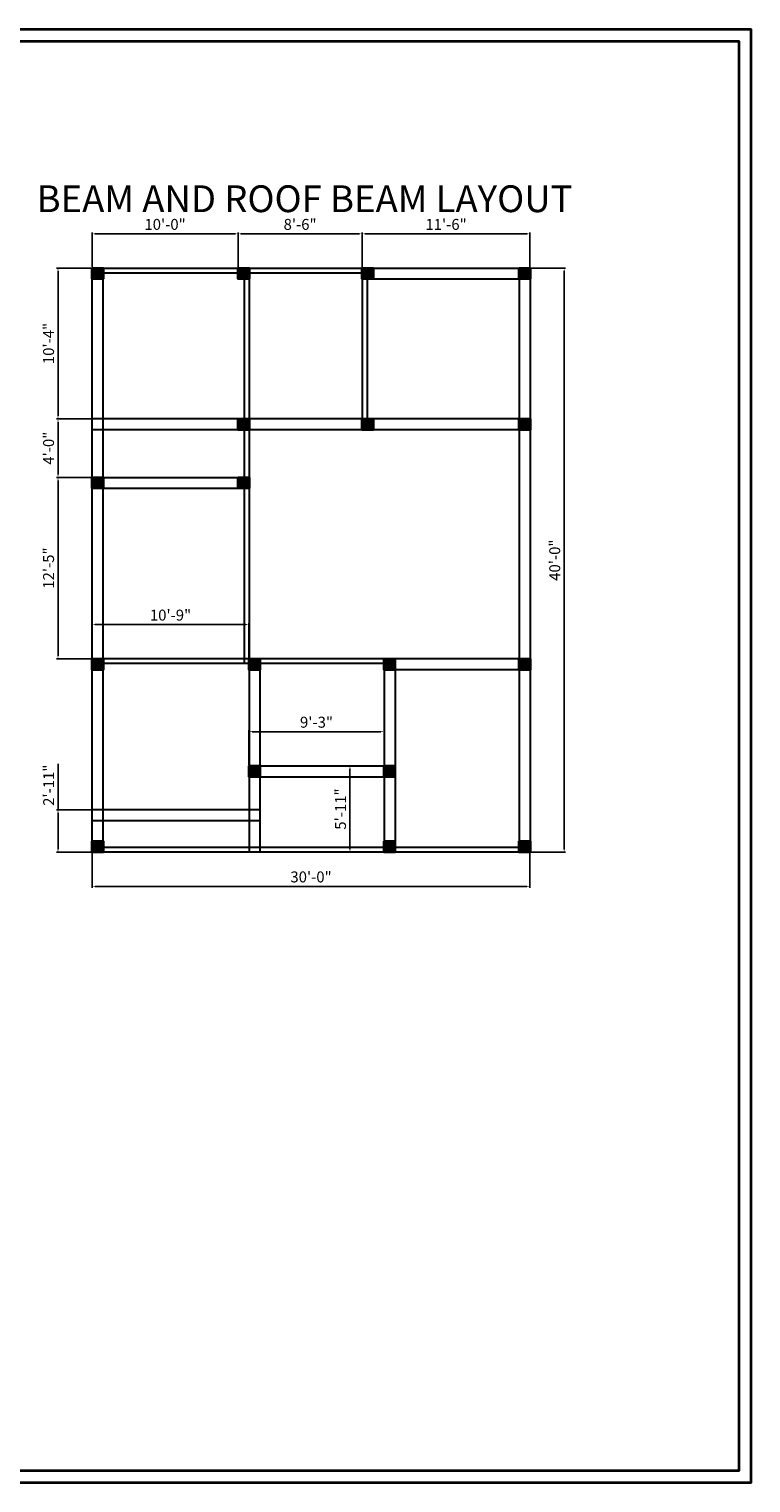
# Model space of a CAD drawing. Units: inches. Extents: x 2413 to 4117, y 1127 to 2321.
# Tile 5 of 5: x 3524 to 4117, y 1127 to 2321. Entities that reach past the tile are written whole.
import ezdxf

# ---------------------------------------------------------------- set-up
doc = ezdxf.new("R2010")
doc.units = ezdxf.units.IN
doc.linetypes.add('ACAD_ISO03W100', pattern=[30, 12, -18])
doc.layers.get('Defpoints').update_dxf_attribs({"linetype": 'ACAD_ISO03W100'})
for name, color, linetype, lineweight in [('A-ANNO-DIMS', 2, 'Continuous', 18), ('A-ANNO-TITL', 7, 'Continuous', 30), ('A-ANNO-TTLB', 7, 'Continuous', 35), ('S-BEAM', 3, 'Continuous', 30), ('S-COLS', 1, 'Continuous', 35)]:
    doc.layers.add(name, color=color, linetype=linetype, lineweight=lineweight)
doc.styles.get("Standard").update_dxf_attribs({"font": 'arial.ttf'})
doc.dimstyles.new('ISO-25', dxfattribs={"dimtxt": 9, "dimasz": 2.5, "dimexe": 1.25, "dimexo": 0.625, "dimgap": 2, "dimtad": 1, "dimdec": 1, "dimlunit": 4, "dimtxsty": 'Standard', "dimcen": 2.5, "dimazin": 0, "dimtfac": 1, "dimtdec": 1, "dimtmove": 0, "dimatfit": 3, "dimfxl": 1, "dimarcsym": 0})

# ---------------------------------------------------------------- blocks, each defined once
blk = doc.blocks.new('COLUMN')
h = blk.add_hatch(color=256)
h.dxf.hatch_style = 1
h.paths.add_polyline_path([(3657, 1935.4), (3666, 1935.4), (3666, 1944.4), (3657, 1944.4)])
blk.add_lwpolyline([(3657, 1944.4), (3666, 1944.4), (3666, 1935.4), (3657, 1935.4)], close=True)
blk = doc.blocks.new('*D54')
at = {"layer": 'A-ANNO-DIMS', "color": 0, "lineweight": -2, "transparency": 16777216}
for p, q in [((3575.4, 2125.7), (3575.4, 2154.3)), ((3577.9, 2153.1), (3692.9, 2153.1)), ((3695.4, 2125.7), (3695.4, 2154.3))]:
    blk.add_line(p, q, dxfattribs=at)
at = {"layer": 'A-ANNO-DIMS', "color": 0, "transparency": 16777216}
for points in [[(3577.9, 2153.5), (3577.9, 2152.7), (3575.4, 2153.1)], [(3692.9, 2153.5), (3692.9, 2152.7), (3695.4, 2153.1)]]:
    blk.add_solid(points, dxfattribs=at)
at = {"layer": 'Defpoints', "color": 0, "transparency": 16777216}
for p in [(3695.4, 2153.1), (3575.4, 2125), (3695.4, 2125)]:
    blk.add_point(p, dxfattribs=at)
at = {"layer": 'A-ANNO-DIMS', "color": 0, "transparency": 16777216, "insert": (3635.4, 2159.7), "char_height": 9, "attachment_point": 5}
blk.add_mtext('10\'-0"', dxfattribs=at)
blk = doc.blocks.new('*D55')
at = {"layer": 'A-ANNO-DIMS', "color": 0, "lineweight": -2, "transparency": 16777216}
for p, q in [((3695.4, 2125.7), (3695.4, 2154.3)), ((3697.9, 2153.1), (3794.9, 2153.1)), ((3797.4, 2125.7), (3797.4, 2154.3))]:
    blk.add_line(p, q, dxfattribs=at)
at = {"layer": 'A-ANNO-DIMS', "color": 0, "transparency": 16777216}
for points in [[(3697.9, 2153.5), (3697.9, 2152.7), (3695.4, 2153.1)], [(3794.9, 2153.5), (3794.9, 2152.7), (3797.4, 2153.1)]]:
    blk.add_solid(points, dxfattribs=at)
at = {"layer": 'Defpoints', "color": 0, "transparency": 16777216}
for p in [(3797.4, 2153.1), (3695.4, 2125), (3797.4, 2125)]:
    blk.add_point(p, dxfattribs=at)
at = {"layer": 'A-ANNO-DIMS', "color": 0, "transparency": 16777216, "insert": (3746.4, 2159.7), "char_height": 9, "attachment_point": 5}
blk.add_mtext('8\'-6"', dxfattribs=at)
blk = doc.blocks.new('*D56')
at = {"layer": 'A-ANNO-DIMS', "color": 0, "lineweight": -2, "transparency": 16777216}
for p, q in [((3797.4, 2125.7), (3797.4, 2154.3)), ((3799.9, 2153.1), (3932.9, 2153.1)), ((3935.4, 2125.7), (3935.4, 2154.3))]:
    blk.add_line(p, q, dxfattribs=at)
at = {"layer": 'A-ANNO-DIMS', "color": 0, "transparency": 16777216}
for points in [[(3799.9, 2153.5), (3799.9, 2152.7), (3797.4, 2153.1)], [(3932.9, 2153.5), (3932.9, 2152.7), (3935.4, 2153.1)]]:
    blk.add_solid(points, dxfattribs=at)
at = {"layer": 'Defpoints', "color": 0, "transparency": 16777216}
for p in [(3935.4, 2153.1), (3797.4, 2125), (3935.4, 2125)]:
    blk.add_point(p, dxfattribs=at)
at = {"layer": 'A-ANNO-DIMS', "color": 0, "transparency": 16777216, "insert": (3866.4, 2159.7), "char_height": 9, "attachment_point": 5}
blk.add_mtext('11\'-6"', dxfattribs=at)
blk = doc.blocks.new('*D57')
at = {"layer": 'A-ANNO-DIMS', "color": 0, "lineweight": -2, "transparency": 16777216}
for p, q in [((3575.4, 1804.7), (3575.4, 1833.3)), ((3577.9, 1832.1), (3701.9, 1832.1)), ((3704.4, 1804.7), (3704.4, 1833.3))]:
    blk.add_line(p, q, dxfattribs=at)
at = {"layer": 'A-ANNO-DIMS', "color": 0, "transparency": 16777216}
for points in [[(3577.9, 1832.5), (3577.9, 1831.7), (3575.4, 1832.1)], [(3701.9, 1832.5), (3701.9, 1831.7), (3704.4, 1832.1)]]:
    blk.add_solid(points, dxfattribs=at)
at = {"layer": 'Defpoints', "color": 0, "transparency": 16777216}
for p in [(3704.4, 1832.1), (3575.4, 1804), (3704.4, 1804)]:
    blk.add_point(p, dxfattribs=at)
at = {"layer": 'A-ANNO-DIMS', "color": 0, "transparency": 16777216, "insert": (3639.9, 1838.7), "char_height": 9, "attachment_point": 5}
blk.add_mtext('10\'-9"', dxfattribs=at)
blk = doc.blocks.new('*D58')
at = {"layer": 'A-ANNO-DIMS', "color": 0, "lineweight": -2, "transparency": 16777216}
for p, q in [((3704.4, 1716.7), (3704.4, 1745.3)), ((3706.9, 1744.1), (3812.9, 1744.1)), ((3815.4, 1716.7), (3815.4, 1745.3))]:
    blk.add_line(p, q, dxfattribs=at)
at = {"layer": 'A-ANNO-DIMS', "color": 0, "transparency": 16777216}
for points in [[(3706.9, 1744.5), (3706.9, 1743.7), (3704.4, 1744.1)], [(3812.9, 1744.5), (3812.9, 1743.7), (3815.4, 1744.1)]]:
    blk.add_solid(points, dxfattribs=at)
at = {"layer": 'Defpoints', "color": 0, "transparency": 16777216}
for p in [(3815.4, 1744.1), (3704.4, 1716), (3815.4, 1716)]:
    blk.add_point(p, dxfattribs=at)
at = {"layer": 'A-ANNO-DIMS', "color": 0, "transparency": 16777216, "insert": (3759.9, 1750.7), "char_height": 9, "attachment_point": 5}
blk.add_mtext('9\'-3"', dxfattribs=at)
blk = doc.blocks.new('*D59')
at = {"layer": 'A-ANNO-DIMS', "color": 0, "lineweight": -2, "transparency": 16777216}
for p, q in [((3547.4, 1680), (3547.4, 1717.6)), ((3574.8, 1680), (3546.1, 1680)), ((3547.4, 1647.5), (3547.4, 1677.5)), ((3574.8, 1645), (3546.1, 1645))]:
    blk.add_line(p, q, dxfattribs=at)
at = {"layer": 'A-ANNO-DIMS', "color": 0, "transparency": 16777216}
for points in [[(3547, 1677.5), (3547.8, 1677.5), (3547.4, 1680)], [(3547, 1647.5), (3547.8, 1647.5), (3547.4, 1645)]]:
    blk.add_solid(points, dxfattribs=at)
at = {"layer": 'Defpoints', "color": 0, "transparency": 16777216}
for p in [(3547.4, 1680), (3575.4, 1680), (3575.4, 1645)]:
    blk.add_point(p, dxfattribs=at)
at = {"layer": 'A-ANNO-DIMS', "color": 0, "transparency": 16777216, "insert": (3540.9, 1700.1), "char_height": 9, "attachment_point": 5, "rotation": 90}
blk.add_mtext('2\'-11"', dxfattribs=at)
blk = doc.blocks.new('*D60')
at = {"layer": 'A-ANNO-DIMS', "color": 0, "lineweight": -2, "transparency": 16777216}
for p, q in [((3814.8, 1716), (3786.1, 1716)), ((3787.4, 1647.5), (3787.4, 1713.5)), ((3814.8, 1645), (3786.1, 1645))]:
    blk.add_line(p, q, dxfattribs=at)
at = {"layer": 'A-ANNO-DIMS', "color": 0, "transparency": 16777216}
for points in [[(3787, 1713.5), (3787.8, 1713.5), (3787.4, 1716)], [(3787, 1647.5), (3787.8, 1647.5), (3787.4, 1645)]]:
    blk.add_solid(points, dxfattribs=at)
at = {"layer": 'Defpoints', "color": 0, "transparency": 16777216}
for p in [(3787.4, 1716), (3815.4, 1716), (3815.4, 1645)]:
    blk.add_point(p, dxfattribs=at)
at = {"layer": 'A-ANNO-DIMS', "color": 0, "transparency": 16777216, "insert": (3780.8, 1680.5), "char_height": 9, "attachment_point": 5, "rotation": 90}
blk.add_mtext('5\'-11"', dxfattribs=at)
blk = doc.blocks.new('*D61')
at = {"layer": 'A-ANNO-DIMS', "color": 0, "lineweight": -2, "transparency": 16777216}
for p, q in [((3574.8, 2125), (3546.1, 2125)), ((3547.4, 2122.5), (3547.4, 2003.5)), ((3574.8, 2001), (3546.1, 2001))]:
    blk.add_line(p, q, dxfattribs=at)
at = {"layer": 'A-ANNO-DIMS', "color": 0, "transparency": 16777216}
for points in [[(3547, 2122.5), (3547.8, 2122.5), (3547.4, 2125)], [(3547, 2003.5), (3547.8, 2003.5), (3547.4, 2001)]]:
    blk.add_solid(points, dxfattribs=at)
at = {"layer": 'Defpoints', "color": 0, "transparency": 16777216}
for p in [(3575.4, 2125), (3547.4, 2001), (3575.4, 2001)]:
    blk.add_point(p, dxfattribs=at)
at = {"layer": 'A-ANNO-DIMS', "color": 0, "transparency": 16777216, "insert": (3540.8, 2063), "char_height": 9, "attachment_point": 5, "rotation": 90}
blk.add_mtext('10\'-4"', dxfattribs=at)
blk = doc.blocks.new('*D62')
at = {"layer": 'A-ANNO-DIMS', "color": 0, "lineweight": -2, "transparency": 16777216}
for p, q in [((3574.8, 2001), (3546.1, 2001)), ((3547.4, 1998.5), (3547.4, 1955.5)), ((3574.8, 1953), (3546.1, 1953))]:
    blk.add_line(p, q, dxfattribs=at)
at = {"layer": 'A-ANNO-DIMS', "color": 0, "transparency": 16777216}
for points in [[(3547, 1998.5), (3547.8, 1998.5), (3547.4, 2001)], [(3547, 1955.5), (3547.8, 1955.5), (3547.4, 1953)]]:
    blk.add_solid(points, dxfattribs=at)
at = {"layer": 'Defpoints', "color": 0, "transparency": 16777216}
for p in [(3575.4, 2001), (3547.4, 1953), (3575.4, 1953)]:
    blk.add_point(p, dxfattribs=at)
at = {"layer": 'A-ANNO-DIMS', "color": 0, "transparency": 16777216, "insert": (3540.8, 1977), "char_height": 9, "attachment_point": 5, "rotation": 90}
blk.add_mtext('4\'-0"', dxfattribs=at)
blk = doc.blocks.new('*D63')
at = {"layer": 'A-ANNO-DIMS', "color": 0, "lineweight": -2, "transparency": 16777216}
for p, q in [((3574.8, 1953), (3546.1, 1953)), ((3547.4, 1950.5), (3547.4, 1806.5)), ((3574.8, 1804), (3546.1, 1804))]:
    blk.add_line(p, q, dxfattribs=at)
at = {"layer": 'A-ANNO-DIMS', "color": 0, "transparency": 16777216}
for points in [[(3547, 1950.5), (3547.8, 1950.5), (3547.4, 1953)], [(3547, 1806.5), (3547.8, 1806.5), (3547.4, 1804)]]:
    blk.add_solid(points, dxfattribs=at)
at = {"layer": 'Defpoints', "color": 0, "transparency": 16777216}
for p in [(3575.4, 1953), (3547.4, 1804), (3575.4, 1804)]:
    blk.add_point(p, dxfattribs=at)
at = {"layer": 'A-ANNO-DIMS', "color": 0, "transparency": 16777216, "insert": (3540.8, 1878.5), "char_height": 9, "attachment_point": 5, "rotation": 90}
blk.add_mtext('12\'-5"', dxfattribs=at)
blk = doc.blocks.new('*D64')
at = {"layer": 'A-ANNO-DIMS', "color": 0, "lineweight": -2, "transparency": 16777216}
for p, q in [((3575.4, 1644.4), (3575.4, 1615.7)), ((3935.4, 1644.4), (3935.4, 1615.7)), ((3577.9, 1617), (3932.9, 1617))]:
    blk.add_line(p, q, dxfattribs=at)
at = {"layer": 'A-ANNO-DIMS', "color": 0, "transparency": 16777216}
for points in [[(3577.9, 1617.4), (3577.9, 1616.6), (3575.4, 1617)], [(3932.9, 1617.4), (3932.9, 1616.6), (3935.4, 1617)]]:
    blk.add_solid(points, dxfattribs=at)
at = {"layer": 'Defpoints', "color": 0, "transparency": 16777216}
for p in [(3575.4, 1645), (3935.4, 1645), (3935.4, 1617)]:
    blk.add_point(p, dxfattribs=at)
at = {"layer": 'A-ANNO-DIMS', "color": 0, "transparency": 16777216, "insert": (3755.4, 1623.6), "char_height": 9, "attachment_point": 5}
blk.add_mtext('30\'-0"', dxfattribs=at)
blk = doc.blocks.new('*D65')
at = {"layer": 'A-ANNO-DIMS', "color": 0, "lineweight": -2, "transparency": 16777216}
for p, q in [((3936.1, 2125), (3964.7, 2125)), ((3963.5, 2122.5), (3963.5, 1647.5)), ((3936.1, 1645), (3964.7, 1645))]:
    blk.add_line(p, q, dxfattribs=at)
at = {"layer": 'A-ANNO-DIMS', "color": 0, "transparency": 16777216}
for points in [[(3963.1, 2122.5), (3963.9, 2122.5), (3963.5, 2125)], [(3963.1, 1647.5), (3963.9, 1647.5), (3963.5, 1645)]]:
    blk.add_solid(points, dxfattribs=at)
at = {"layer": 'Defpoints', "color": 0, "transparency": 16777216}
for p in [(3935.4, 2125), (3935.4, 1645), (3963.5, 1645)]:
    blk.add_point(p, dxfattribs=at)
at = {"layer": 'A-ANNO-DIMS', "color": 0, "transparency": 16777216, "insert": (3956.9, 1885), "char_height": 9, "attachment_point": 5, "rotation": 90}
blk.add_mtext('40\'-0"', dxfattribs=at)

msp = doc.modelspace()

# ---------------------------------------------------------------- linework, layer by layer
at = {"layer": 'A-ANNO-TTLB'}
for points in [[(2412.62, 2321.32), (4117.04, 2321.32), (4117.04, 1126.9), (2412.62, 1126.9)], [(2422.62, 2311.32), (4107.04, 2311.32), (4107.04, 1136.9), (2422.62, 1136.9)]]:
    msp.add_lwpolyline(points, close=True, dxfattribs=at)
at = {"layer": 'S-BEAM'}
for p, q in [((3575.43, 2125.03), (3935.43, 2125.03)), ((3575.43, 1645.03), (3575.43, 2125.03)), ((3575.43, 2116.03), (3584.43, 2116.03)), ((3584.43, 1645.03), (3584.43, 2125.03)), ((3584.43, 2121.03), (3797.43, 2121.03)), ((3695.43, 2116.03), (3704.43, 2116.03)), ((3700.43, 2116.03), (3700.43, 2001.03)), ((3704.43, 2125.03), (3704.43, 1645.03)), ((3797.43, 2121.03), (3797.43, 1992.03)), ((3797.43, 2116.03), (3935.43, 2116.03)), ((3801.43, 2116.03), (3801.43, 2001.03)), ((3926.43, 2125.03), (3926.43, 1645.03)), ((3935.43, 2125.03), (3935.43, 1645.03)), ((3935.43, 2001.03), (3575.43, 2001.03)), ((3935.43, 1992.03), (3575.43, 1992.03)), ((3700.43, 1992.03), (3700.43, 1800.03)), ((3575.43, 1953.03), (3704.43, 1953.03)), ((3575.43, 1944.03), (3704.43, 1944.03)), ((3935.43, 1804.03), (3575.43, 1804.03)), ((3713.43, 1804.03), (3713.43, 1645.03)), ((3815.43, 1804.03), (3815.43, 1645.03)), ((3824.43, 1804.03), (3824.43, 1645.03)), ((3584.43, 1795.03), (3575.43, 1795.03)), ((3704.43, 1800.03), (3584.43, 1800.03)), ((3713.43, 1795.03), (3704.43, 1795.03)), ((3815.43, 1800.03), (3713.43, 1800.03)), ((3935.43, 1795.03), (3815.43, 1795.03)), ((3704.43, 1716.03), (3824.43, 1716.03)), ((3704.43, 1707.03), (3824.43, 1707.03)), ((3575.43, 1680.03), (3713.43, 1680.03)), ((3575.43, 1671.03), (3713.43, 1671.03)), ((3584.43, 1654.03), (3575.43, 1654.03)), ((3926.43, 1649.03), (3584.43, 1649.03)), ((3935.43, 1645.03), (3575.43, 1645.03))]:
    msp.add_line(p, q, dxfattribs=at)

# ---------------------------------------------------------------- block references
at = {"layer": 'S-COLS'}
for p in [(-81.59, 180.62), (38.41, 180.62), (140.41, 180.62), (269.41, 180.62), (38.41, 56.62), (140.41, 56.62), (269.41, 56.62), (-81.59, 8.62), (38.41, 8.62), (-81.59, -140.38), (47.41, -140.38), (158.41, -140.38), (269.41, -140.38), (47.41, -228.38), (158.41, -228.38), (-81.59, -290.38), (158.41, -290.38), (269.41, -290.38)]:
    msp.add_blockref('COLUMN', p, dxfattribs=at)

# ---------------------------------------------------------------- texts
at = {"layer": 'A-ANNO-TITL'}
msp.add_text('BEAM AND ROOF BEAM LAYOUT', height=22.0248, dxfattribs=at).set_placement((3529.8, 2170.92))

# ---------------------------------------------------------------- dimensions: what is measured, and where the dimension line sits
at = {"layer": 'A-ANNO-DIMS'}
for base, p1, p2, picture, middle in [((3695.43, 2153.08), (3575.43, 2125.03), (3695.43, 2125.03), '*D54', (3635.43, 2159.68)), ((3797.43, 2153.08), (3695.43, 2125.03), (3797.43, 2125.03), '*D55', (3746.43, 2159.68)), ((3935.43, 2153.08), (3797.43, 2125.03), (3935.43, 2125.03), '*D56', (3866.43, 2159.68)), ((3935.43, 1616.98), (3575.43, 1645.03), (3935.43, 1645.03), '*D64', (3755.43, 1623.58))]:
    dim = msp.add_linear_dim(base=base, p1=p1, p2=p2, dimstyle='ISO-25', override={"dimdec": 1, "dimlfac": 1, "dimrnd": 0, "dimzin": 1, "dimdsep": 46, "dimlunit": 4, "dimfrac": 2}, dxfattribs=at)
    dim.commit()
    dim.dimension.update_dxf_attribs({"geometry": picture, "text_midpoint": middle})
for base, p1, p2, angle, picture, middle in [((3547.38, 2001.03), (3575.43, 2125.03), (3575.43, 2001.03), 90, '*D61', (3540.79, 2063.03)), ((3963.48, 1645.03), (3935.43, 2125.03), (3935.43, 1645.03), 90, '*D65', (3956.89, 1885.03)), ((3547.38, 1953.03), (3575.43, 2001.03), (3575.43, 1953.03), 90, '*D62', (3540.79, 1977.03)), ((3547.38, 1804.03), (3575.43, 1953.03), (3575.43, 1804.03), 90, '*D63', (3540.79, 1878.53)), ((3704.43, 1832.08), (3575.43, 1804.03), (3704.43, 1804.03), 0, '*D57', (3639.93, 1838.68)), ((3815.43, 1744.08), (3704.43, 1716.03), (3815.43, 1716.03), 0, '*D58', (3759.93, 1750.68)), ((3547.38, 1680.03), (3575.43, 1645.03), (3575.43, 1680.03), 90, '*D59', (3540.86, 1700.07)), ((3787.38, 1716.03), (3815.43, 1645.03), (3815.43, 1716.03), 90, '*D60', (3780.79, 1680.53))]:
    dim = msp.add_linear_dim(base=base, p1=p1, p2=p2, angle=angle, dimstyle='ISO-25', override={"dimdec": 1, "dimlfac": 1, "dimrnd": 0, "dimzin": 1, "dimdsep": 46, "dimlunit": 4, "dimfrac": 2}, dxfattribs=at)
    dim.commit()
    dim.dimension.update_dxf_attribs({"geometry": picture, "text_midpoint": middle})

doc.saveas('drawing.dxf')
